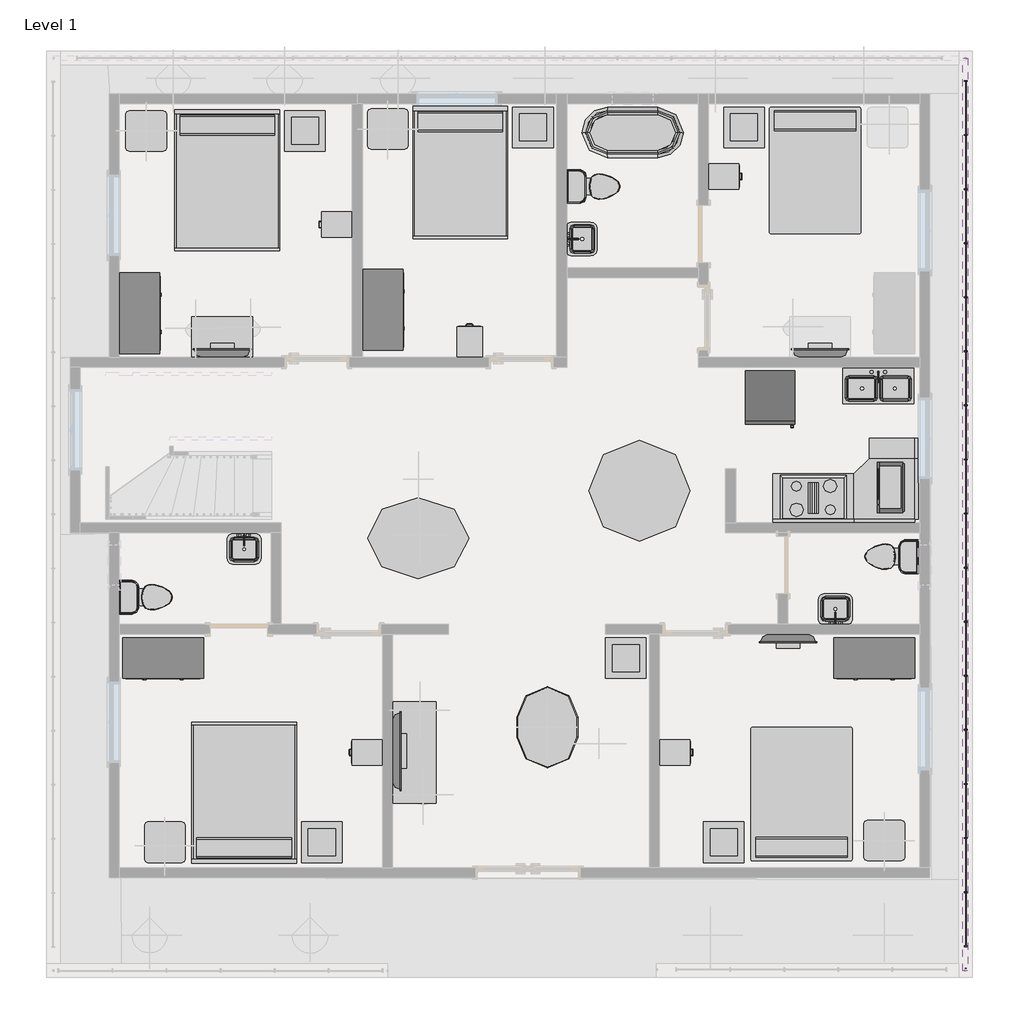
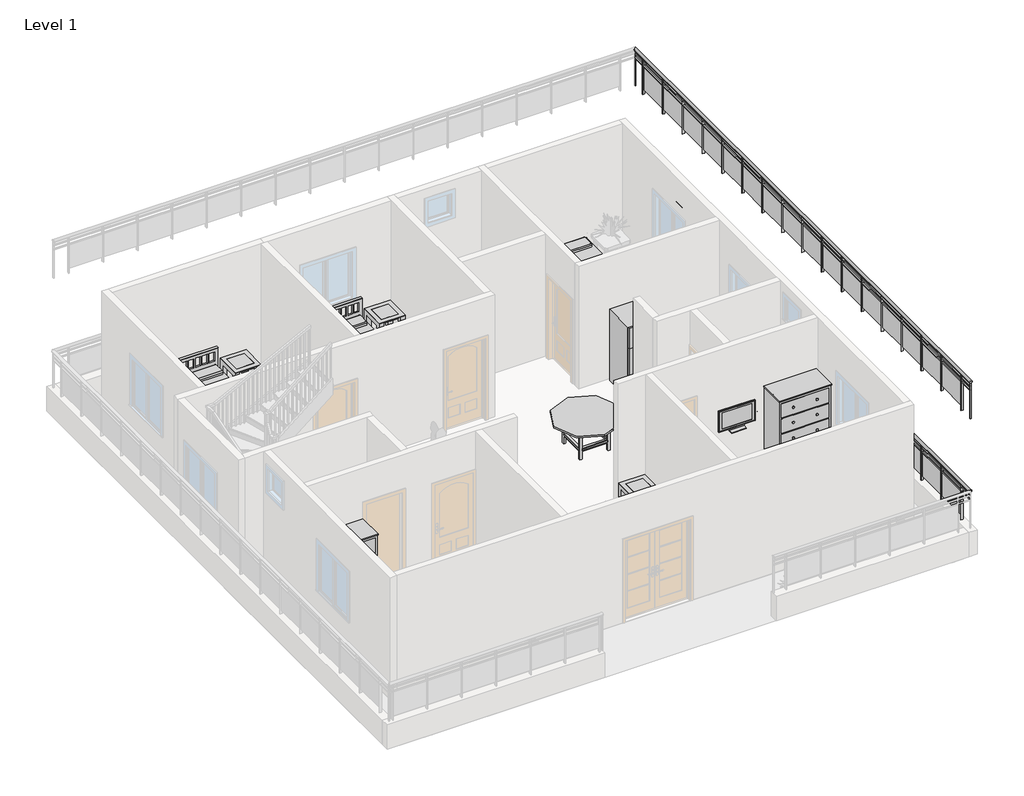
# One storey, part 4 of 5: 34 furniture elements, 11 flow terminals, 3 proxies, 2 railings.
# Revit data of these elements (continued)
# Type "Glass Panel - Bottom Fill" (continued)
#   built-in parameter 1008611 = 0.0416667 (stored number, unit not read)
#   built-in parameter 1008609 = 0.333333 (stored number, unit not read)
#   built-in parameter 1008604 = 0.166667 (stored number, unit not read)
#   built-in parameter 1008603 = 0.166667 (stored number, unit not read)
#   Railing Height = 3' - 0"
#   built-in parameter 1008630 = 2
#   built-in parameter 1008610 = 2
#   built-in parameter 1008618 = Baluster - Square : 3/4"
# Element 1 (IfcBuildingElementProxy, "Cook Top-4 Unit : 36\" x 20\"")
#   Phase Created = New Construction
#   Materials on its faces: "Steel, Chrome Plated", "Steel, Polished"
# Element 2 (IfcBuildingElementProxy, "Microwave : 30\" x 16\" x 18\"")
#   Phase Created = New Construction
#   Materials on its faces: "Laminate, Linen, Matte", "Glass"
# Element 3 (IfcBuildingElementProxy, "Refrigerator : 30\" x 32\" RH")
#   Phase Created = New Construction
#   Materials on its faces: "Carpet (1)", "Steel, Chrome Plated"
# Element 4 (IfcFlowTerminal, "Floor Drain - Round : 5\" Strainer - 2\" Drain")
#   Mark = "4"
#   Phase Created = New Construction
# Element 5 (IfcFlowTerminal, "Floor Drain - Round : 5\" Strainer - 2\" Drain")
#   Mark = "8"
#   Phase Created = New Construction
# Element 6 (IfcFlowTerminal, "Floor Drain - Round : 5\" Strainer - 2\" Drain")
#   Mark = "12"
#   Phase Created = New Construction
# Element 7 (IfcFlowTerminal, "Sink Kitchen-Double : 42\" x 21\"")
#   Mark = "13"
#   Phase Created = New Construction
#   Materials on its faces: "Steel, Polished"
# Element 8 (IfcFlowTerminal, "Sink Vanity-Square : 20\" x 18\"")
#   Mark = "3"
#   Phase Created = New Construction
#   Materials on its faces: "Porcelain, Linen", "Steel, Polished"
# Element 9 (IfcFlowTerminal, "Sink Vanity-Square : 20\" x 18\"")
#   Mark = "9"
#   Phase Created = New Construction
#   Materials on its faces: "Porcelain, Linen", "Steel, Polished"
# Element 10 (IfcFlowTerminal, "Sink Vanity-Square : 20\" x 18\"")
#   Mark = "11"
#   Phase Created = New Construction
#   Materials on its faces: "Porcelain, Linen", "Steel, Polished"
# Element 11 (IfcFlowTerminal, "Toilet-Domestic-3D : Toilet-Domestic-3D")
#   Mark = "2"
#   Phase Created = New Construction
#   Materials on its faces: "Porcelain, Linen", "Laminate, Linen, Matte"
# Element 12 (IfcFlowTerminal, "Toilet-Domestic-3D : Toilet-Domestic-3D")
#   Mark = "6"
#   Phase Created = New Construction
#   Materials on its faces: "Porcelain, Linen", "Laminate, Linen, Matte"
# Element 13 (IfcFlowTerminal, "Toilet-Domestic-3D : Toilet-Domestic-3D")
#   Mark = "10"
#   Phase Created = New Construction
#   Materials on its faces: "Porcelain, Linen", "Laminate, Linen, Matte"
# Element 14 (IfcFlowTerminal, "Tub-Free Standing-3D : 30\" x 60\"")
#   Mark = "1"
#   Phase Created = New Construction
#   Materials on its faces: "Porcelain, Ivory"
# Element 15 (IfcFurniture, "Bed-Shaker : Double 56\" x 78\"")
#   Phase Created = New Construction
#   Materials on its faces: "Birch", "Plywood, Sheathing"
# Elements 16, 17 (IfcFurniture, "Bed-Shaker : Queen 62\" x 83\"")
#   Phase Created = New Construction
#   Materials on its faces: "Birch", "Plywood, Sheathing"
# Element 18 (IfcFurniture, "Bed-Standard : Double 54\" x 75\"")
#   Phase Created = New Construction
#   Materials on its faces: "Linen, White", "Steel, Chrome Plated"
# Element 19 (IfcFurniture, "Bed-Standard : Queen 60\" x 79\"")
#   Phase Created = New Construction
#   Materials on its faces: "Linen, White", "Steel, Chrome Plated"
# Elements 20, 21, 22, 23, 24 (IfcFurniture, "Cabinet-File 2 Drawer : 15\" x 18\"")
#   Phase Created = New Construction
#   Materials on its faces: "Steel, Chrome Plated", "Wood - Teak"
# Elements 25, 26, 27, 28 (IfcFurniture, "Dresser : 48\" x 72\" x 24\"")
#   Phase Created = New Construction
#   Materials on its faces: "Laminate, Ivory, Matte", "Cherry", "Wood - Teak"
# Elements 29, 30, 31 (IfcFurniture, "TV - Flat Screen : 32\"")
#   Stand = yes
#   Phase Created = New Construction
#   Materials on its faces: "TV - Black", "TV - Glass", "TV - Screen"
# Element 32 (IfcFurniture, "TV - Flat Screen : 46\"")
#   Stand = yes
#   Phase Created = New Construction
#   Materials on its faces: "TV - Black", "TV - Glass", "TV - Screen"
# Elements 33, 34, 35, 36, 37, 38 (IfcFurniture, "Table-Coffee : 24\" x 24\" x 24\"")
#   Phase Created = New Construction
#   Materials on its faces: "Paper", "Glass - Clear, Grey"
# Element 39 (IfcFurniture, "Table-Dining Oval : 36\" x 48\"")
#   Phase Created = New Construction
#   Materials on its faces: "Steel, Chrome Plated", "Glass - Clear, Grey"
# Element 40 (IfcFurniture, "Table-Dining Round w Chairs : 60\" Diameter")
#   Phase Created = New Construction
#   Materials on its faces: "Pine", "Wood - Teak"
# Element 41 (IfcFurniture, "Table-Ellipse : 60\" x 48\"")
#   Phase Created = New Construction
#   Materials on its faces: "Birch"
# Elements 42, 43, 44, 45 (IfcFurniture, "Table-End : 24\" x 24\"")
#   Phase Created = New Construction
#   Materials on its faces: "Laminate, Ivory, Matte", "Birch"
# Element 46 (IfcFurniture, "Table-Rectangular : 72\" x 30\"")
#   Phase Created = New Construction
#   Materials on its faces: "Birch"
# Element 47 (IfcFurniture, "Table-Rectangular : 72\" x 30\" 2")
#   Phase Created = New Construction
#   Materials on its faces: "Birch"
# Element 48 (IfcFurniture, "Work Station Cubicle : 96\" x 96\"")
#   Phase Created = New Construction
#   Materials on its faces: "Textile - Light Gray", "Laminate, Ivory, Matte"
# Element 49 (IfcRailing, "Glass Panel - Bottom Fill")
#   built-in parameter 1008621 = 11 (stored number, unit not read)
#   Phase Created = New Construction
#   Materials on its faces: "Glass"
# Element 50 (IfcRailing, "Glass Panel - Bottom Fill")
#   built-in parameter 1008621 = 2 (stored number, unit not read)
#   Phase Created = New Construction
#   Materials on its faces: "Glass"
# Materials
#   "Steel, Chrome Plated": class "Metal", colour RGB 17 17 17, transparency 0, Description = "Chromiuim plated steel", Cost = 0
#   "Steel, Polished": class "Metal", colour RGB 57 57 57, transparency 0, Description = "Polished steel", Cost = 0
#   "Laminate, Linen, Matte": class "Plastic", colour RGB 249 239 230, transparency 0, Description = "Plastic Laminate - Linen, Matte", Cost = 0
#   "Carpet (1)": class "Carpet", colour RGB 124 80 67, transparency 0, Description = "Interior finish"
#   "Porcelain, Linen": class "Ceramic", colour RGB 249 239 230, transparency 0, Description = "Porcelain, linen", Cost = 0
#   "Porcelain, Ivory": class "Ceramic", colour RGB 247 247 239, transparency 0, Description = "Porcelain, ivory", Cost = 0
#   "Birch": class "Wood", colour RGB 224 178 126, transparency 0, Description = "Betula Alleghaniensis", Cost = 0
#   "Plywood, Sheathing": class "Wood", colour RGB 212 179 113, transparency 0, Description = "Plywood, sheathing grade", Cost = 0
#   "Oak Flooring": class "Wood", colour RGB 216 169 114, transparency 0, Description = "Quercus Rubra", Cost = 0
#   "Wood - Teak": class "Wood", colour RGB 145 112 90, transparency 0
#   "Cherry": class "Wood", colour RGB 226 177 128, transparency 0, Description = "Prunus Serotina", Cost = 0
#   "Paper": class "Generic", colour RGB 0 0 0, transparency 0, Description = "Paper", Cost = 0
#   "Glass - Clear, Grey": class "Glass", colour RGB 252 255 255, transparency 0.64
#   "Pine": class "Wood", colour RGB 223 192 134, transparency 0, Description = "Pinus Echinata", Cost = 0
#   "Laminate, Ivory, Matte": class "Plastic", colour RGB 247 247 239, transparency 0, Description = "Plastic Laminate - Ivory, Matte", Cost = 0
#   "Textile - Light Gray": class "Fabric", colour RGB 204 204 204, transparency 0
#   "Glass": class "Glass", colour RGB 0 128 192, transparency 0.75, Description = "Soda Lime Glass", Cost = 0
#   "Linen, White": class "Textile", colour RGB 247 247 239, transparency 0, Description = "Linen, white", Cost = 0
#   "TV - Black": colour RGB 49 49 49, transparency 0
#   "TV - Glass": colour RGB 157 157 157, transparency 0.9
#   "TV - Screen": colour RGB 0 0 0, transparency 0
